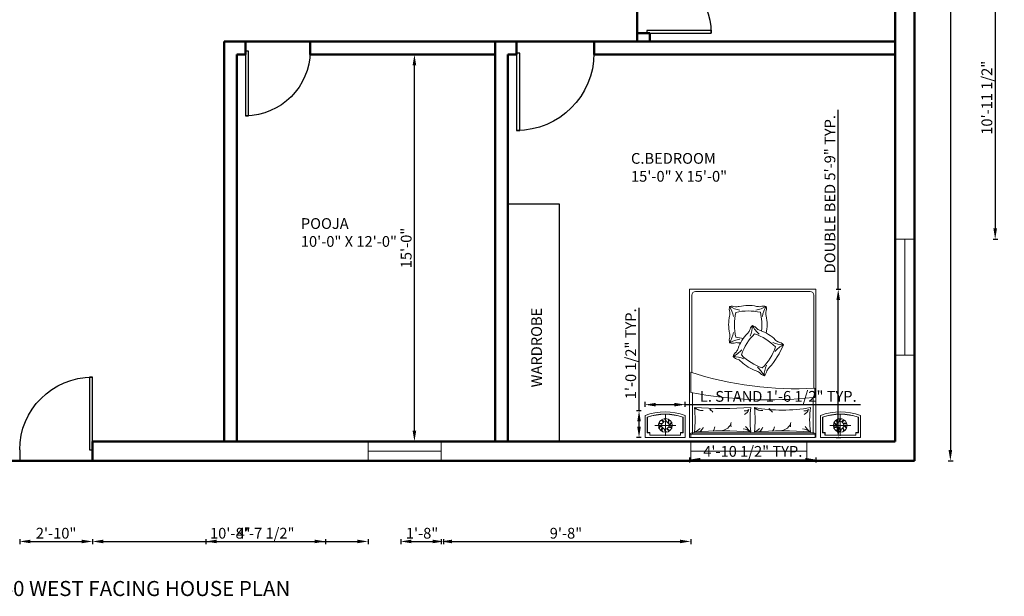
# Model space of a CAD drawing. Units: inches. Extents: x -46 to 764, y -530 to 112.
# Tile 3 of 5: x 307 to 764, y -530 to -262. Entities that reach past the tile are written whole.
import ezdxf

# ---------------------------------------------------------------- set-up
doc = ezdxf.new("R2010")
doc.units = ezdxf.units.IN
for name, color, linetype, lineweight in [('A-ANNO-DIMS', 2, 'Continuous', 18), ('A-AREA-IDEN', 7, 'Continuous', 18), ('A-DOOR', 3, 'Continuous', 25), ('A-FLOR-CASE', 32, 'Continuous', 25), ('A-GLAZ', 4, 'Continuous', 18), ('A-WALL', 7, 'Continuous', 50), ('furn', 28, 'Continuous', 18), ('txt', 167, 'Continuous', 18)]:
    doc.layers.add(name, color=color, linetype=linetype, lineweight=lineweight)
doc.styles.get("Standard").update_dxf_attribs({"font": 'arial.ttf'})
doc.dimstyles.new('ISO-25', dxfattribs={"dimtxt": 5, "dimasz": 5, "dimexe": 1.25, "dimexo": 0.625, "dimtad": 1, "dimlunit": 3, "dimtxsty": 'Standard', "dimcen": 2.5, "dimadec": 0, "dimazin": 0, "dimtfac": 1, "dimtmove": 0, "dimatfit": 3, "dimfxl": 1, "dimfxlon": 1, "dimarcsym": 0})

# ---------------------------------------------------------------- blocks, each defined once
blk = doc.blocks.new('*U2')
for p, q in [((0, 0), (0, -6)), ((40, 0), (40, -6))]:
    blk.add_line(p, q)
blk.add_lwpolyline([(0, 0), (0, 40), (1.75, 40), (1.75, 0)], close=True)
blk.add_arc((0, 0), 40, 0, 90)
blk = doc.blocks.new('*D11')
at = {"layer": 'A-ANNO-DIMS', "color": 0, "lineweight": -2, "transparency": 16777216}
for p, q in [((738.29, 12.97), (740.54, 12.97)), ((739.29, 7.97), (739.29, -462.03)), ((738.29, -467.03), (740.54, -467.03))]:
    blk.add_line(p, q, dxfattribs=at)
at = {"layer": 'A-ANNO-DIMS', "color": 0, "transparency": 16777216}
for points in [[(738.46, 7.97), (740.13, 7.97), (739.29, 12.97)], [(738.46, -462.03), (740.13, -462.03), (739.29, -467.03)]]:
    blk.add_solid(points, dxfattribs=at)
at = {"layer": 'Defpoints', "color": 0, "transparency": 16777216}
for p in [(722.62, 12.97), (722.62, -467.03), (739.29, -467.03)]:
    blk.add_point(p, dxfattribs=at)
at = {"layer": 'A-ANNO-DIMS', "color": 0, "transparency": 16777216, "insert": (736.12, -227.03), "char_height": 5, "attachment_point": 5, "rotation": 90}
blk.add_mtext("40'", dxfattribs=at)
blk = doc.blocks.new('BED-DOUBLE')
for p, q in [((1.34, 1.59), (1.34, 20.76)), ((57.43, 1.59), (57.43, 18.55)), ((57.72, 2.1), (1.02, 2.1))]:
    blk.add_line(p, q)
for points in [[(58.74, 0), (58.74, 68.93), (0, 68.93), (0, 0)], [(0.55, 0), (0.55, 1.59), (58.4, 1.59), (58.4, 0), (0, 0)]]:
    blk.add_lwpolyline(points)
for points in [[(57.72, 22.84), (57.72, 66.21, 0.414214), (56.03, 67.91), (2.72, 67.91, 0.414214), (1.02, 66.21), (1.02, 30.17)], [(18.6, 60.97, 0.159461), (18.72, 58.3, -0.076283), (18.6, 56.51, 0.115075), (18.6, 48.45, -0.076283), (18.72, 46.67, 0.159461), (18.6, 43.99)], [(20.35, 56.21, 0.091296), (18.6, 60.97, 0.091296), (23.37, 59.23)], [(30.8, 59.23, 0.091296), (35.58, 60.97, 0.091296), (33.82, 56.21, 0.091296)], [(32.9, 58.2, 0.111006), (21.48, 58.19, 0.119549), (21.48, 46.63, 0.033212), (24.99, 46.09)], [(29.21, 52.07, 0.159461), (27.9, 49.74, -0.076283), (26.85, 48.29, 0.115075), (22.59, 41.45, -0.076283), (21.75, 39.87, 0.159461), (20.23, 37.66)], [(28.18, 47.1, 0.091296), (29.21, 52.07, 0.091296), (32.34, 48.07)], [(23.37, 45.73, 0.091296), (18.6, 43.99, 0.091296), (20.35, 48.76, 0.091296)], [(39.88, 42.16, 0.111006), (30.18, 48.19, 0.119549), (24.07, 38.38, 0.107813), (33.74, 32.32)], [(33.79, 32.33, 0.121865), (39.88, 42.16, 0.121865)], [(38.65, 44.14, 0.091296), (43.62, 43.09, 0.091296), (39.61, 39.98, 0.091296)], [(25.2, 36.61, 0.091296), (20.23, 37.66, 0.091296), (24.24, 40.78, 0.091296)], [(35.68, 33.66, 0.091296), (34.64, 28.68, 0.091296), (31.51, 32.68, 0.091296)]]:
    blk.add_lwpolyline(points, format="xyb")
for points in [[(58.23, 18.55), (57.43, 18.55, -0.072944), (0.55, 20.92), (0.55, 30.34, 0.092568), (58.23, 22.87)], [(28.45, 13.91, 0.058596), (28.45, 2.57, 0.036648), (2.28, 2.57, 0.052163), (2.28, 13.91, 0.036967)], [(56.14, 13.91, 0.058596), (56.14, 2.57, 0.036889), (30.14, 2.57, 0.052163), (30.14, 13.91, 0.093111)]]:
    blk.add_lwpolyline(points, format="xyb", close=True)
for centre, radius, start, end in [((19.65, 56.16), 4.92, 70.7023, 102.284), ((21.76, 66.68), 5.9, 265.2252, 282.6741), ((27.14, 43.67), 17.74, 77.0576, 103.3153), ((32.37, 66.72), 5.9, 257.6988, 275.1477), ((34.43, 56.82), 4.3, 74.5791, 110.8198), ((31.43, 59.81), 4.3, 339.3666, 15.6073), ((9.55, 52.37), 24.07, 353.1956, 14.0284), ((41.33, 57.79), 5.9, 175.0387, 192.4877), ((18.3, 52.48), 17.74, 346.8711, 13.1289), ((27.56, 47.43), 4.92, 38.7754, 70.3571), ((34.92, 55.25), 5.9, 233.2983, 250.7472), ((27.31, 32.87), 17.74, 45.1307, 71.3884), ((19.87, 47.76), 3.97, 251.3996, 291.5774), ((21.86, 38.19), 5.9, 77.6988, 95.1477), ((27.09, 61.25), 17.74, 257.0576, 258.7033), ((9.2, 57.16), 37.18, 318.3818, 337.7644), ((43.94, 49.66), 5.9, 225.7718, 243.2208), ((40.46, 40.18), 4.3, 42.6522, 78.8929), ((23.3, 40.19), 3.97, 219.4726, 259.6505), ((19.93, 31.02), 5.9, 45.7718, 63.2208), ((36.56, 47.81), 17.74, 225.1307, 251.3884), ((41.21, 28.34), 5.9, 135.5854, 153.0343), ((28.95, 25.44), 5.9, 53.2983, 70.7472), ((35.78, 32.68), 4.15, 217.2937, 254.0973), ((31.74, 31.86), 4.3, 312.4658, 348.7065), ((4.9, 15.54), 2.94, 213.6349, 270.8456), ((5.76, 17.16), 4.64, 224.406, 276.8342), ((33.45, 17.16), 4.64, 224.406, 276.8342), ((32.59, 15.54), 2.94, 213.6349, 270.8456), ((10.31, 13.43), 0.952, 173.7543, 257.2187), ((20.8, 21.81), 14.18, 216.2085, 225.0849), ((25.94, 14.96), 2.58, 256.4823, 308.5563), ((23.98, 14.17), 3.77, 294.2916, 340.9896), ((38, 13.43), 0.952, 173.7543, 257.2187), ((48.49, 21.81), 14.18, 216.2085, 225.0849), ((53.63, 14.96), 2.58, 256.4823, 308.5563), ((51.67, 14.17), 3.77, 294.2916, 340.9896), ((1.84, 6.34), 4.75, 310.5354, 340.3558), ((7.42, 5.72), 4.41, 321.8174, 349.8987), ((13.79, 9.29), 6.29, 276.6849, 328.3182), ((21.96, 5.79), 2.82, 155.8927, 196.1192), ((36.96, 13.18), 13.6, 216.4935, 231.2792), ((29.53, 6.34), 4.75, 310.5354, 340.3558), ((35.11, 5.72), 4.41, 321.8174, 349.8987), ((41.48, 9.29), 6.29, 276.6849, 328.3182), ((49.65, 5.79), 2.82, 155.8927, 196.1192), ((64.65, 13.18), 13.6, 216.4935, 231.2792), ((1.02, 1.08), 1.02, 90, 180), ((-1.12, 10.34), 8.56, 294.6457, 314.1585), ((22.41, -6.92), 11.24, 57.5379, 77.5233), ((26.57, 10.34), 8.56, 294.6457, 314.1585), ((50.1, -6.92), 11.24, 57.5379, 77.5233), ((57.72, 1.08), 1.02, 0, 90)]:
    blk.add_arc(centre, radius, start, end)
blk = doc.blocks.new('NIGHTSTAND-L')
for p, q in [((9.43, 10.52), (9.43, 0.73)), ((4.54, 5.63), (14.33, 5.63))]:
    blk.add_line(p, q)
blk.add_lwpolyline([(0, 10.19), (0, 0), (18.68, 0), (18.68, 10.19, 0.181818)], format="xyb", close=True)
for points in [[(17.66, 2.14), (17.66, 9.48, 0.167087), (1.02, 9.48), (1.02, 2.14)], [(17.55, 2.14), (17.55, 9.4, 0.165559), (1.12, 9.4), (1.12, 2.14)]]:
    blk.add_lwpolyline(points, format="xyb")
for points in [[(2.24, 1.02), (2.24, 2.24), (1.02, 2.24)], [(2.14, 1.02), (2.14, 2.14), (1.02, 2.14)], [(2.14, 1.12), (16.54, 1.12)], [(2.14, 1.02), (16.54, 1.02)], [(16.43, 1.02), (16.43, 2.24), (17.66, 2.24)], [(16.54, 1.02), (16.54, 2.14), (17.66, 2.14)]]:
    blk.add_lwpolyline(points)
for radius in [3.2, 1.73]:
    blk.add_circle((9.43, 5.63), radius)
for centre, radius, start, end in [((6.99, 4.73), 1.57, 67.462, 127.6998), ((7.01, 4.53), 2.05, 69.5103, 115.83), ((8.02, 3.43), 2.05, 105.5103, 151.83), ((7.89, 3.59), 1.57, 103.462, 163.6998), ((7.17, 6.28), 1.57, 31.462, 91.6998), ((7.07, 6.1), 2.05, 33.5103, 79.83), ((7.98, 7.48), 1.57, 355.462, 55.6998), ((7.8, 7.4), 2.05, 357.5103, 43.83), ((9.35, 7.98), 1.57, 319.462, 19.6998), ((9.15, 8.02), 2.05, 321.5103, 7.83), ((11.63, 6.64), 2.05, 249.5103, 295.83), ((11.64, 6.43), 1.57, 247.462, 307.6998), ((10.75, 7.58), 1.57, 283.462, 343.6998), ((10.61, 7.73), 2.05, 285.5103, 331.83), ((9.48, 3.14), 2.05, 141.5103, 187.83), ((9.52, 3.28), 1.57, 139.462, 199.6998), ((11.07, 3.86), 2.05, 177.5103, 223.83), ((10.88, 3.77), 1.57, 175.462, 235.6998), ((11.8, 5.16), 2.05, 213.5103, 259.83), ((11.7, 4.98), 1.57, 211.462, 271.6998)]:
    blk.add_arc(centre, radius, start, end)
blk = doc.blocks.new('NIGHTSTAND-R')
for p, q in [((9.24, 10.52), (9.24, 0.73)), ((14.14, 5.62), (4.35, 5.62))]:
    blk.add_line(p, q)
blk.add_lwpolyline([(18.68, 10.19), (18.68, 0), (0, 0), (0, 10.19, -0.181818)], format="xyb", close=True)
for points in [[(1.02, 2.14), (1.02, 9.48, -0.167087), (17.66, 9.48), (17.66, 2.14)], [(1.12, 2.14), (1.12, 9.4, -0.165559), (17.56, 9.4), (17.56, 2.14)]]:
    blk.add_lwpolyline(points, format="xyb")
for points in [[(2.24, 1.02), (2.24, 2.24), (1.02, 2.24)], [(2.14, 1.02), (2.14, 2.14), (1.02, 2.14)], [(16.54, 1.12), (2.14, 1.12)], [(16.54, 1.02), (2.14, 1.02)], [(16.43, 1.02), (16.43, 2.24), (17.66, 2.24)], [(16.54, 1.02), (16.54, 2.14), (17.66, 2.14)]]:
    blk.add_lwpolyline(points)
for radius in [3.2, 1.73]:
    blk.add_circle((9.24, 5.62), radius)
for centre, radius, start, end in [((7.03, 6.43), 1.57, 232.3002, 292.538), ((7.05, 6.63), 2.05, 244.17, 290.4897), ((8.06, 7.73), 2.05, 208.17, 254.4897), ((7.93, 7.57), 1.57, 196.3002, 256.538), ((9.52, 8.02), 2.05, 172.17, 218.4897), ((9.32, 7.97), 1.57, 160.3002, 220.538), ((10.88, 7.4), 2.05, 136.17, 182.4897), ((10.69, 7.48), 1.57, 124.3002, 184.538), ((11.61, 6.09), 2.05, 100.17, 146.4897), ((11.5, 6.27), 1.57, 88.3002, 148.538), ((11.43, 4.61), 2.05, 64.17, 110.4897), ((11.45, 4.82), 1.57, 52.3002, 112.538), ((10.56, 3.67), 1.57, 16.3002, 76.538), ((10.42, 3.52), 2.05, 28.17, 74.4897), ((6.98, 4.98), 1.57, 268.3002, 328.538), ((6.88, 5.15), 2.05, 280.17, 326.4897), ((7.79, 3.77), 1.57, 304.3002, 4.538), ((7.6, 3.85), 2.05, 316.17, 2.4897), ((9.16, 3.27), 1.57, 340.3002, 40.538), ((8.96, 3.23), 2.05, 352.17, 38.4897)]:
    blk.add_arc(centre, radius, start, end)
blk = doc.blocks.new('WIN-54IN')
blk.add_line((4.5, 54), (4.5, 0))
blk.add_lwpolyline([(0, 54), (9, 54), (9, 0), (0, 0)], close=True)
blk = doc.blocks.new('WIN-34IN')
blk.add_line((0, 4.5), (34, 4.5))
blk.add_lwpolyline([(0, 9), (34, 9), (34, 0), (0, 0)], close=True)
blk = doc.blocks.new('*D27')
at = {"layer": 'A-ANNO-DIMS', "color": 0, "lineweight": -2, "transparency": 16777216}
for p, q in [((687.15, -387.22), (687.15, -303.78)), ((686.15, -387.22), (688.4, -387.22)), ((687.15, -451.15), (687.15, -392.22)), ((686.15, -456.15), (688.4, -456.15))]:
    blk.add_line(p, q, dxfattribs=at)
at = {"layer": 'A-ANNO-DIMS', "color": 0, "transparency": 16777216}
for points in [[(686.32, -392.22), (687.98, -392.22), (687.15, -387.22)], [(686.32, -451.15), (687.98, -451.15), (687.15, -456.15)]]:
    blk.add_solid(points, dxfattribs=at)
at = {"layer": 'Defpoints', "color": 0, "transparency": 16777216}
for p in [(676.81, -387.22), (687.15, -387.22), (676.81, -456.15)]:
    blk.add_point(p, dxfattribs=at)
at = {"layer": 'A-ANNO-DIMS', "color": 0, "transparency": 16777216, "insert": (683.94, -343), "char_height": 5, "attachment_point": 5, "rotation": 90}
blk.add_mtext('DOUBLE BED 5\'-9" TYP.', dxfattribs=at)
blk = doc.blocks.new('*D28')
at = {"layer": 'A-ANNO-DIMS', "color": 0, "lineweight": -2, "transparency": 16777216}
for p, q in [((618.07, -465.49), (618.07, -467.74)), ((623.07, -466.49), (671.81, -466.49)), ((676.81, -465.49), (676.81, -467.74))]:
    blk.add_line(p, q, dxfattribs=at)
at = {"layer": 'A-ANNO-DIMS', "color": 0, "transparency": 16777216}
for points in [[(623.07, -465.66), (623.07, -467.33), (618.07, -466.49)], [(671.81, -465.66), (671.81, -467.33), (676.81, -466.49)]]:
    blk.add_solid(points, dxfattribs=at)
at = {"layer": 'Defpoints', "color": 0, "transparency": 16777216}
for p in [(618.07, -456.15), (676.81, -456.15), (676.81, -466.49)]:
    blk.add_point(p, dxfattribs=at)
at = {"layer": 'A-ANNO-DIMS', "color": 0, "transparency": 16777216, "insert": (647.44, -463.28), "char_height": 5, "attachment_point": 5}
blk.add_mtext('4\'-10 1/2" TYP.', dxfattribs=at)
blk = doc.blocks.new('*D29')
at = {"layer": 'A-ANNO-DIMS', "color": 0, "lineweight": -2, "transparency": 16777216}
for p, q in [((597.35, -441.9), (597.35, -439.65)), ((602.35, -440.9), (611.03, -440.9)), ((616.03, -441.9), (616.03, -439.65)), ((616.03, -440.9), (697.57, -440.9))]:
    blk.add_line(p, q, dxfattribs=at)
at = {"layer": 'A-ANNO-DIMS', "color": 0, "transparency": 16777216}
for points in [[(602.35, -440.07), (602.35, -441.73), (597.35, -440.9)], [(611.03, -440.07), (611.03, -441.73), (616.03, -440.9)]]:
    blk.add_solid(points, dxfattribs=at)
at = {"layer": 'Defpoints', "color": 0, "transparency": 16777216}
for p in [(597.35, -443.7), (616.03, -440.9), (616.03, -443.7)]:
    blk.add_point(p, dxfattribs=at)
at = {"layer": 'A-ANNO-DIMS', "color": 0, "transparency": 16777216, "insert": (659.3, -437.69), "char_height": 5, "attachment_point": 5}
blk.add_mtext('L. STAND 1\'-6 1/2" TYP.', dxfattribs=at)
blk = doc.blocks.new('*D30')
at = {"layer": 'A-ANNO-DIMS', "color": 0, "lineweight": -2, "transparency": 16777216}
for p, q in [((594.55, -443.7), (594.55, -395.79)), ((595.55, -443.7), (593.3, -443.7)), ((594.55, -451.15), (594.55, -448.7)), ((595.55, -456.15), (593.3, -456.15))]:
    blk.add_line(p, q, dxfattribs=at)
at = {"layer": 'A-ANNO-DIMS', "color": 0, "transparency": 16777216}
for points in [[(593.72, -448.7), (595.39, -448.7), (594.55, -443.7)], [(593.72, -451.15), (595.39, -451.15), (594.55, -456.15)]]:
    blk.add_solid(points, dxfattribs=at)
at = {"layer": 'Defpoints', "color": 0, "transparency": 16777216}
for p in [(594.55, -443.7), (597.35, -443.7), (597.35, -456.15)]:
    blk.add_point(p, dxfattribs=at)
at = {"layer": 'A-ANNO-DIMS', "color": 0, "transparency": 16777216, "insert": (591.34, -417.25), "char_height": 5, "attachment_point": 5, "rotation": 90}
blk.add_mtext('1\'-0 1/2" TYP.', dxfattribs=at)
blk = doc.blocks.new('*D40')
at = {"layer": 'A-ANNO-DIMS', "color": 0, "lineweight": -2, "transparency": 16777216}
for p, q in [((483.74, -503.53), (483.74, -505.78)), ((503.62, -503.53), (503.62, -505.78)), ((488.74, -504.53), (498.62, -504.53))]:
    blk.add_line(p, q, dxfattribs=at)
at = {"layer": 'A-ANNO-DIMS', "color": 0, "transparency": 16777216}
for points in [[(488.74, -503.7), (488.74, -505.36), (483.74, -504.53)], [(498.62, -503.7), (498.62, -505.36), (503.62, -504.53)]]:
    blk.add_solid(points, dxfattribs=at)
at = {"layer": 'Defpoints', "color": 0, "transparency": 16777216}
for p in [(483.74, -135.15), (503.62, -135.15), (503.62, -504.53)]:
    blk.add_point(p, dxfattribs=at)
at = {"layer": 'A-ANNO-DIMS', "color": 0, "transparency": 16777216, "insert": (493.68, -501.35), "char_height": 5, "attachment_point": 5}
blk.add_mtext('1\'-8"', dxfattribs=at)
blk = doc.blocks.new('*D41')
at = {"layer": 'A-ANNO-DIMS', "color": 0, "lineweight": -2, "transparency": 16777216}
for p, q in [((393.18, -503.53), (393.18, -505.78)), ((448.74, -503.53), (448.74, -505.78)), ((398.18, -504.53), (443.74, -504.53))]:
    blk.add_line(p, q, dxfattribs=at)
at = {"layer": 'A-ANNO-DIMS', "color": 0, "transparency": 16777216}
for points in [[(398.18, -503.7), (398.18, -505.36), (393.18, -504.53)], [(443.74, -503.7), (443.74, -505.36), (448.74, -504.53)]]:
    blk.add_solid(points, dxfattribs=at)
at = {"layer": 'Defpoints', "color": 0, "transparency": 16777216}
for p in [(393.18, -72.15), (448.74, -72.15), (448.74, -504.53)]:
    blk.add_point(p, dxfattribs=at)
at = {"layer": 'A-ANNO-DIMS', "color": 0, "transparency": 16777216, "insert": (420.96, -501.32), "char_height": 5, "attachment_point": 5}
blk.add_mtext('4\'-7 1/2"', dxfattribs=at)
blk = doc.blocks.new('*D61')
at = {"layer": 'A-ANNO-DIMS', "color": 0, "lineweight": -2, "transparency": 16777216}
for p, q in [((759.12, -232.39), (761.37, -232.39)), ((760.12, -237.39), (760.12, -358.93)), ((759.12, -363.93), (761.37, -363.93))]:
    blk.add_line(p, q, dxfattribs=at)
at = {"layer": 'A-ANNO-DIMS', "color": 0, "transparency": 16777216}
for points in [[(759.29, -237.39), (760.96, -237.39), (760.12, -232.39)], [(759.29, -358.93), (760.96, -358.93), (760.12, -363.93)]]:
    blk.add_solid(points, dxfattribs=at)
at = {"layer": 'Defpoints', "color": 0, "transparency": 16777216}
for p in [(722.62, -232.39), (722.62, -363.93), (760.12, -363.93)]:
    blk.add_point(p, dxfattribs=at)
at = {"layer": 'A-ANNO-DIMS', "color": 0, "transparency": 16777216, "insert": (756.91, -298.16), "char_height": 5, "attachment_point": 5, "rotation": 90}
blk.add_mtext('10\'-11 1/2"', dxfattribs=at)
blk = doc.blocks.new('*D65')
at = {"layer": 'A-ANNO-DIMS', "color": 0, "lineweight": -2, "transparency": 16777216}
for p, q in [((306.62, -503.53), (306.62, -505.78)), ((340.48, -503.53), (340.48, -505.78)), ((311.62, -504.53), (335.48, -504.53))]:
    blk.add_line(p, q, dxfattribs=at)
at = {"layer": 'A-ANNO-DIMS', "color": 0, "transparency": 16777216}
for points in [[(311.62, -503.7), (311.62, -505.36), (306.62, -504.53)], [(335.48, -503.7), (335.48, -505.36), (340.48, -504.53)]]:
    blk.add_solid(points, dxfattribs=at)
at = {"layer": 'Defpoints', "color": 0, "transparency": 16777216}
for p in [(306.62, -467.03), (340.48, -467.03), (340.48, -504.53)]:
    blk.add_point(p, dxfattribs=at)
at = {"layer": 'A-ANNO-DIMS', "color": 0, "transparency": 16777216, "insert": (323.55, -501.35), "char_height": 5, "attachment_point": 5}
blk.add_mtext('2\'-10"', dxfattribs=at)
blk = doc.blocks.new('*D66')
at = {"layer": 'A-ANNO-DIMS', "color": 0, "lineweight": -2, "transparency": 16777216}
for p, q in [((340.48, -503.53), (340.48, -505.78)), ((468.56, -503.53), (468.56, -505.78)), ((345.48, -504.53), (463.56, -504.53))]:
    blk.add_line(p, q, dxfattribs=at)
at = {"layer": 'A-ANNO-DIMS', "color": 0, "transparency": 16777216}
for points in [[(345.48, -503.7), (345.48, -505.36), (340.48, -504.53)], [(463.56, -503.7), (463.56, -505.36), (468.56, -504.53)]]:
    blk.add_solid(points, dxfattribs=at)
at = {"layer": 'Defpoints', "color": 0, "transparency": 16777216}
for p in [(340.48, -467.03), (468.56, -467.03), (468.56, -504.53)]:
    blk.add_point(p, dxfattribs=at)
at = {"layer": 'A-ANNO-DIMS', "color": 0, "transparency": 16777216, "insert": (404.52, -501.35), "char_height": 5, "attachment_point": 5}
blk.add_mtext('10\'-8"', dxfattribs=at)
blk = doc.blocks.new('*D67')
at = {"layer": 'A-ANNO-DIMS', "color": 0, "lineweight": -2, "transparency": 16777216}
for p, q in [((502.56, -503.53), (502.56, -505.78)), ((618.59, -503.53), (618.59, -505.78)), ((507.56, -504.53), (613.59, -504.53))]:
    blk.add_line(p, q, dxfattribs=at)
at = {"layer": 'A-ANNO-DIMS', "color": 0, "transparency": 16777216}
for points in [[(507.56, -503.7), (507.56, -505.36), (502.56, -504.53)], [(613.59, -503.7), (613.59, -505.36), (618.59, -504.53)]]:
    blk.add_solid(points, dxfattribs=at)
at = {"layer": 'Defpoints', "color": 0, "transparency": 16777216}
for p in [(502.56, -467.03), (618.59, -467.01), (618.59, -504.53)]:
    blk.add_point(p, dxfattribs=at)
at = {"layer": 'A-ANNO-DIMS', "color": 0, "transparency": 16777216, "insert": (560.58, -501.35), "char_height": 5, "attachment_point": 5}
blk.add_mtext('9\'-8"', dxfattribs=at)
blk = doc.blocks.new('*D76')
at = {"layer": 'A-ANNO-DIMS', "color": 0, "lineweight": -2, "transparency": 16777216}
for p, q in [((411.62, 100.72), (411.62, 102.97)), ((416.62, 101.72), (436.62, 101.72)), ((441.62, 100.72), (441.62, 102.97))]:
    blk.add_line(p, q, dxfattribs=at)
at = {"layer": 'A-ANNO-DIMS', "color": 0, "transparency": 16777216}
for points in [[(416.62, 102.55), (416.62, 100.88), (411.62, 101.72)], [(436.62, 102.55), (436.62, 100.88), (441.62, 101.72)]]:
    blk.add_solid(points, dxfattribs=at)
at = {"layer": 'Defpoints', "color": 0, "transparency": 16777216}
for p in [(441.62, 101.72), (411.62, -272.03), (441.62, -272.03)]:
    blk.add_point(p, dxfattribs=at)
at = {"layer": 'A-ANNO-DIMS', "color": 0, "transparency": 16777216, "insert": (426.62, 104.89), "char_height": 5, "attachment_point": 5}
blk.add_mtext('2\'-6"', dxfattribs=at)
blk = doc.blocks.new('*D77')
at = {"layer": 'A-ANNO-DIMS', "color": 0, "lineweight": -2, "transparency": 16777216}
for p, q in [((537.62, 100.72), (537.62, 102.97)), ((542.62, 101.72), (568.62, 101.72)), ((573.62, 100.72), (573.62, 102.97))]:
    blk.add_line(p, q, dxfattribs=at)
at = {"layer": 'A-ANNO-DIMS', "color": 0, "transparency": 16777216}
for points in [[(542.62, 102.55), (542.62, 100.88), (537.62, 101.72)], [(568.62, 102.55), (568.62, 100.88), (573.62, 101.72)]]:
    blk.add_solid(points, dxfattribs=at)
at = {"layer": 'Defpoints', "color": 0, "transparency": 16777216}
for p in [(573.62, 101.72), (537.62, -272.03), (573.62, -272.03)]:
    blk.add_point(p, dxfattribs=at)
at = {"layer": 'A-ANNO-DIMS', "color": 0, "transparency": 16777216, "insert": (555.62, 104.9), "char_height": 5, "attachment_point": 5}
blk.add_mtext('3\'-0"', dxfattribs=at)
blk = doc.blocks.new('*D78')
at = {"layer": 'A-ANNO-DIMS', "color": 0, "lineweight": -2, "transparency": 16777216}
for p, q in [((245.34, 100.72), (245.34, 102.97)), ((250.34, 101.72), (396.62, 101.72)), ((401.62, 100.72), (401.62, 102.97))]:
    blk.add_line(p, q, dxfattribs=at)
at = {"layer": 'A-ANNO-DIMS', "color": 0, "transparency": 16777216}
for points in [[(250.34, 102.55), (250.34, 100.88), (245.34, 101.72)], [(396.62, 102.55), (396.62, 100.88), (401.62, 101.72)]]:
    blk.add_solid(points, dxfattribs=at)
at = {"layer": 'Defpoints', "color": 0, "transparency": 16777216}
for p in [(401.62, 101.72), (245.34, -458.03), (401.62, -458.03)]:
    blk.add_point(p, dxfattribs=at)
at = {"layer": 'A-ANNO-DIMS', "color": 0, "transparency": 16777216, "insert": (323.48, 104.93), "char_height": 5, "attachment_point": 5}
blk.add_mtext('13\'-0 1/2"', dxfattribs=at)
blk = doc.blocks.new('*D79')
at = {"layer": 'A-ANNO-DIMS', "color": 0, "lineweight": -2, "transparency": 16777216}
for p, q in [((491.12, -278.03), (488.87, -278.03)), ((490.12, -453.03), (490.12, -283.03)), ((491.12, -458.03), (488.87, -458.03))]:
    blk.add_line(p, q, dxfattribs=at)
at = {"layer": 'A-ANNO-DIMS', "color": 0, "transparency": 16777216}
for points in [[(489.29, -283.03), (490.96, -283.03), (490.12, -278.03)], [(489.29, -453.03), (490.96, -453.03), (490.12, -458.03)]]:
    blk.add_solid(points, dxfattribs=at)
at = {"layer": 'Defpoints', "color": 0, "transparency": 16777216}
for p in [(490.12, -278.03), (527.62, -278.03), (527.62, -458.03)]:
    blk.add_point(p, dxfattribs=at)
at = {"layer": 'A-ANNO-DIMS', "color": 0, "transparency": 16777216, "insert": (486.95, -368.03), "char_height": 5, "attachment_point": 5, "rotation": 90}
blk.add_mtext('15\'-0"', dxfattribs=at)

msp = doc.modelspace()

# ---------------------------------------------------------------- linework, layer by layer
at = {"layer": 'A-FLOR-CASE'}
for p, q in [((557.624, -347.692), (533.624, -347.692)), ((557.624, -458.03), (557.624, -347.692))]:
    msp.add_line(p, q, dxfattribs=at)
at = {"layer": 'A-WALL'}
for p, q in [((722.624, 12.97), (722.624, -467.03)), ((713.624, 3.97), (713.624, -458.03)), ((593.624, -182.03), (593.624, -272.03)), ((599.624, -268.107), (593.624, -268.107)), ((599.624, -268.107), (599.624, -272.03)), ((401.624, -272.03), (527.624, -272.03)), ((401.624, -278.03), (401.624, -272.03)), ((411.624, -278.03), (411.624, -272.03)), ((441.624, -278.03), (441.624, -272.03)), ((527.624, -272.03), (713.624, -272.03)), ((527.624, -278.03), (527.624, -272.03)), ((537.624, -278.03), (537.624, -272.03)), ((573.624, -278.03), (573.624, -272.03)), ((401.624, -458.03), (401.624, -278.03)), ((407.624, -458.03), (407.624, -278.03)), ((407.624, -278.03), (411.624, -278.03)), ((441.624, -278.03), (527.624, -278.03)), ((527.624, -458.03), (527.624, -278.03)), ((533.624, -458.03), (533.624, -278.03)), ((533.624, -278.03), (537.624, -278.03)), ((573.624, -278.03), (713.624, -278.03)), ((713.624, -458.03), (340.481, -458.03)), ((340.481, -458.03), (340.481, -467.03)), ((722.624, -467.03), (2.624, -467.03))]:
    msp.add_line(p, q, dxfattribs=at)

# ---------------------------------------------------------------- block references
at = {"layer": 'A-DOOR'}
for p, xscale, yscale, zscale, rotation in [((598.119, -268.107), -0.7492007242236776, 0.7492007242236776, 0.7492007242236776, 270), ((411.624, -276.525), -0.749131318087898, 0.749131318087898, 0.749131318087898, 180), ((537.624, -277.428), -0.8996712828794231, 0.8996712828794231, 0.8996712828794231, 180)]:
    msp.add_blockref('*U2', p, dxfattribs=dict(at, xscale=xscale, yscale=yscale, zscale=zscale, rotation=rotation))
at = {"layer": 'A-DOOR', "xscale": -0.8466483010861098, "yscale": 0.8466483010861098, "zscale": 0.8466483010861098}
msp.add_blockref('*U2', (340.481, -461.95), dxfattribs=at)
at = {"layer": 'A-GLAZ'}
for name, p in [('WIN-54IN', (713.624, -417.925)), ('WIN-34IN', (468.561, -467.03))]:
    msp.add_blockref(name, p, dxfattribs=at)
at = {"layer": 'A-GLAZ', "rotation": 269.9999999999999}
msp.add_blockref('WIN-54IN', (618.592, -458.008), dxfattribs=at)
at = {"layer": 'furn'}
for name, p in [('BED-DOUBLE', (618.068, -456.153)), ('NIGHTSTAND-L', (597.355, -456.152)), ('NIGHTSTAND-R', (678.848, -456.149))]:
    msp.add_blockref(name, p, dxfattribs=at)

# ---------------------------------------------------------------- texts
at = {"layer": 'A-AREA-IDEN', "char_height": 5, "attachment_point": 1}
for s, width, insert in [('C.BEDROOM\\P15\'-0" X 15\'-0"', 73.09773, (590.823, -323.86)), ('POOJA\\P10\'-0" X 12\'-0"', 75.59494, (437.327, -354.157))]:
    msp.add_mtext_dynamic_manual_height_columns(s, width=width, gutter_width=12.5, heights=[0], dxfattribs=dict(at, insert=insert))
at = {"layer": 'txt', "insert": (544.421, -432.884), "char_height": 5, "attachment_point": 1, "rotation": 90}
msp.add_mtext_dynamic_manual_height_columns('WARDROBE', width=154.75533, gutter_width=12.5, heights=[0], dxfattribs=at)
at = {"layer": 'txt', "insert": (282.157, -522.92), "char_height": 7, "attachment_point": 1}
msp.add_mtext_dynamic_manual_height_columns('60X40 WEST FACING HOUSE PLAN', width=376.83273, gutter_width=12.5, heights=[0], dxfattribs=at)

# ---------------------------------------------------------------- dimensions: what is measured, and where the dimension line sits
at = {"layer": 'A-ANNO-DIMS'}
for base, p1, p2, picture, middle in [((401.624, 101.716), (245.339, -458.03), (401.624, -458.03), '*D78', (323.481, 104.928)), ((441.624, 101.716), (411.624, -272.03), (441.624, -272.03), '*D76', (426.624, 104.894)), ((573.624, 101.716), (537.624, -272.03), (573.624, -272.03), '*D77', (555.624, 104.896)), ((448.744, -504.53), (393.176, -72.153), (448.744, -72.153), '*D41', (420.96, -501.319)), ((503.624, -504.53), (483.741, -135.15), (503.624, -135.15), '*D40', (493.682, -501.352)), ((340.481, -504.53), (306.615, -467.03), (340.481, -467.03), '*D65', (323.548, -501.352)), ((468.562, -504.53), (340.481, -467.03), (468.562, -467.03), '*D66', (404.522, -501.352)), ((618.592, -504.53), (502.562, -467.03), (618.592, -467.008), '*D67', (560.577, -501.352))]:
    dim = msp.add_linear_dim(base=base, p1=p1, p2=p2, dimstyle='ISO-25', override={"dimdec": 1, "dimlfac": 1, "dimrnd": 0, "dimzin": 1, "dimdsep": 46, "dimlunit": 4, "dimfrac": 2}, dxfattribs=at)
    dim.commit()
    dim.dimension.update_dxf_attribs({"geometry": picture, "text_midpoint": middle})
for base, p1, p2, override, picture, middle in [((739.294, -467.03), (722.624, 12.97), (722.624, -467.03), {"dimclrd": 0, "dimclre": 0, "dimclrt": 0}, '*D11', (736.116, -227.03)), ((760.124, -363.925), (722.624, -232.39), (722.624, -363.925), {"dimdec": 1, "dimlfac": 1, "dimrnd": 0, "dimzin": 1, "dimdsep": 46, "dimlunit": 4, "dimfrac": 2}, '*D61', (756.914, -298.157)), ((490.124, -278.03), (527.624, -458.03), (527.624, -278.03), {"dimdec": 1, "dimlfac": 1, "dimrnd": 0, "dimzin": 1, "dimdsep": 46, "dimlunit": 4, "dimfrac": 2}, '*D79', (486.946, -368.03))]:
    dim = msp.add_linear_dim(base=base, p1=p1, p2=p2, angle=90, dimstyle='ISO-25', override=override, dxfattribs=at)
    dim.commit()
    dim.dimension.update_dxf_attribs({"geometry": picture, "text_midpoint": middle})
for base, p1, p2, text, picture, middle in [((687.151, -387.224), (676.811, -456.154), (676.811, -387.224), 'DOUBLE BED <> TYP.', '*D27', (683.939, -343.001)), ((594.554, -443.702), (597.355, -456.153), (597.355, -443.702), '<> TYP.', '*D30', (591.343, -417.249))]:
    dim = msp.add_linear_dim(base=base, p1=p1, p2=p2, angle=90, text=text, dimstyle='ISO-25', override={"dimdec": 1, "dimlfac": 1, "dimrnd": 0, "dimzin": 1, "dimdsep": 46, "dimlunit": 4, "dimfrac": 2}, dxfattribs=at)
    dim.commit()
    dim.dimension.update_dxf_attribs({"geometry": picture, "text_midpoint": middle})
for base, p1, p2, text, picture, middle in [((616.03, -440.901), (597.355, -443.702), (616.03, -443.702), 'L. STAND <> TYP.', '*D29', (659.299, -437.691)), ((676.811, -466.493), (618.068, -456.154), (676.811, -456.154), '<> TYP.', '*D28', (647.439, -463.283))]:
    dim = msp.add_linear_dim(base=base, p1=p1, p2=p2, text=text, dimstyle='ISO-25', override={"dimdec": 1, "dimlfac": 1, "dimrnd": 0, "dimzin": 1, "dimdsep": 46, "dimlunit": 4, "dimfrac": 2}, dxfattribs=at)
    dim.commit()
    dim.dimension.update_dxf_attribs({"geometry": picture, "text_midpoint": middle})

doc.saveas('drawing.dxf')
